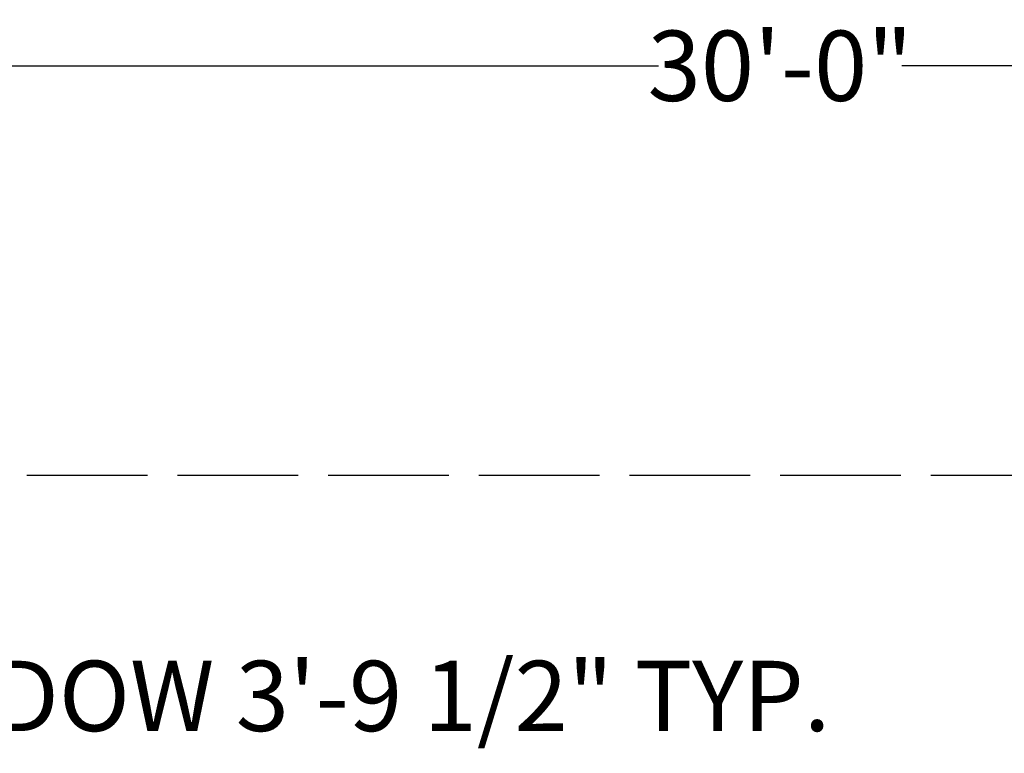
# Model space of a CAD drawing. Units: inches. Extents: x 1316 to 1777, y 813 to 1650.
# Tile 14 of 22: x 1469 to 1567, y 1576 to 1650. Entities that reach past the tile are written whole.
import ezdxf

# ---------------------------------------------------------------- set-up
doc = ezdxf.new("R2010")
doc.units = ezdxf.units.IN
doc.header["$MEASUREMENT"] = 0
doc.linetypes.add('ACAD_ISO02W100', pattern=[15, 12, -3])
doc.layers.add('A-ANNO-DIMS', color=2, linetype='Continuous', lineweight=18)
doc.layers.add('C-PROP', color=8, linetype='ACAD_ISO02W100', lineweight=25)
doc.styles.get("Standard").update_dxf_attribs({"font": 'arial.ttf'})
doc.dimstyles.get("Standard").update_dxf_attribs({"dimtxt": 7, "dimasz": 0.18, "dimexe": 0.18, "dimexo": 0.0625, "dimgap": 0.09, "dimtad": 0, "dimtih": 1, "dimtoh": 1, "dimzin": 0, "dimdsep": 46, "dimlunit": 3, "dimtxsty": 'Standard', "dimcen": 0.09, "dimadec": 0, "dimazin": 0, "dimtfac": 1, "dimtofl": 0, "dimtmove": 0, "dimatfit": 3, "dimfxl": 1, "dimtolj": 1, "dimtzin": 0, "dimarcsym": 0})

# ---------------------------------------------------------------- blocks, each defined once
blk = doc.blocks.new('*D22')
at = {"layer": 'A-ANNO-DIMS', "color": 0, "lineweight": -2, "transparency": 16777216}
for p, q in [((1364.398563382318, 1644.458857483655), (1364.398563382318, 1645.129391375627)), ((1364.578563382317, 1644.949391375628), (1532.287758470994, 1644.949391375628)), ((1724.218563382317, 1644.949391375628), (1556.509368293641, 1644.949391375628)), ((1724.398563382317, 1644.458857483655), (1724.398563382317, 1645.129391375627))]:
    blk.add_line(p, q, dxfattribs=at)
at = {"layer": 'A-ANNO-DIMS', "color": 0, "transparency": 16777216}
for points in [[(1364.578563382317, 1644.979391375628), (1364.578563382317, 1644.919391375628), (1364.398563382318, 1644.949391375628)], [(1724.218563382317, 1644.979391375628), (1724.218563382317, 1644.919391375628), (1724.398563382317, 1644.949391375628)]]:
    blk.add_solid(points, dxfattribs=at)
at = {"layer": 'Defpoints', "color": 0, "transparency": 16777216}
for p in [(1724.398563382317, 1644.949391375628), (1364.398563382318, 1644.396357483655), (1724.398563382317, 1644.396357483655)]:
    blk.add_point(p, dxfattribs=at)
at = {"layer": 'A-ANNO-DIMS', "color": 0, "transparency": 16777216, "insert": (1544.398563382318, 1644.949391375628), "char_height": 7, "attachment_point": 5}
blk.add_mtext('\\A1;30\'-0"', dxfattribs=at)
blk = doc.blocks.new('*D34')
at = {"layer": 'A-ANNO-DIMS', "color": 0, "lineweight": -2, "transparency": 16777216}
for p, q in [((1400.4446139869, 1575.431800926962), (1400.4446139869, 1582.375827866596)), ((1400.6246139869, 1582.195827866596), (1445.774793584458, 1582.195827866596)), ((1445.954793584458, 1575.431800926962), (1445.954793584458, 1582.375827866596)), ((1445.954793584458, 1582.195827866596), (1446.134793584458, 1582.195827866596))]:
    blk.add_line(p, q, dxfattribs=at)
at = {"layer": 'A-ANNO-DIMS', "color": 0, "transparency": 16777216}
for points in [[(1400.6246139869, 1582.225827866596), (1400.6246139869, 1582.165827866596), (1400.4446139869, 1582.195827866596)], [(1445.774793584458, 1582.225827866596), (1445.774793584458, 1582.165827866596), (1445.954793584458, 1582.195827866596)]]:
    blk.add_solid(points, dxfattribs=at)
at = {"layer": 'Defpoints', "color": 0, "transparency": 16777216}
for p in [(1445.954793584458, 1582.195827866596), (1400.4446139869, 1575.369300926962), (1445.954793584458, 1575.369300926962)]:
    blk.add_point(p, dxfattribs=at)
at = {"layer": 'A-ANNO-DIMS', "color": 0, "transparency": 16777216, "insert": (1498.669882261129, 1582.195827866596), "char_height": 7, "attachment_point": 5}
blk.add_mtext('\\A1;WINDOW 3\'-9 1/2" TYP.', dxfattribs=at)

msp = doc.modelspace()

# ---------------------------------------------------------------- linework, layer by layer
at = {"layer": 'C-PROP'}
msp.add_line((1364.398563382318, 1604.172951843256), (1724.398563382317, 1604.172951843256), dxfattribs=at)

# ---------------------------------------------------------------- dimensions: what is measured, and where the dimension line sits
at = {"layer": 'A-ANNO-DIMS'}
for base, p1, p2, text, override, picture, middle in [((1724.398563382317, 1644.949391375628), (1364.398563382318, 1644.396357483655), (1724.398563382317, 1644.396357483655), '30\'-0"', {"dimclrd": 0, "dimclre": 0, "dimclrt": 0}, '*D22', (1544.398563382318, 1644.949391375628)), ((1445.954793584458, 1582.195827866596), (1400.4446139869, 1575.369300926962), (1445.954793584458, 1575.369300926962), 'WINDOW <> TYP.', {"dimdec": 1, "dimlfac": 1, "dimrnd": 0, "dimzin": 1, "dimdsep": 46, "dimlunit": 4, "dimfrac": 2}, '*D34', (1498.669882261129, 1582.195827866596))]:
    dim = msp.add_linear_dim(base=base, p1=p1, p2=p2, text=text, dimstyle='Standard', override=override, dxfattribs=at)
    dim.commit()
    dim.dimension.update_dxf_attribs({"geometry": picture, "text_midpoint": middle})

doc.saveas('drawing.dxf')
